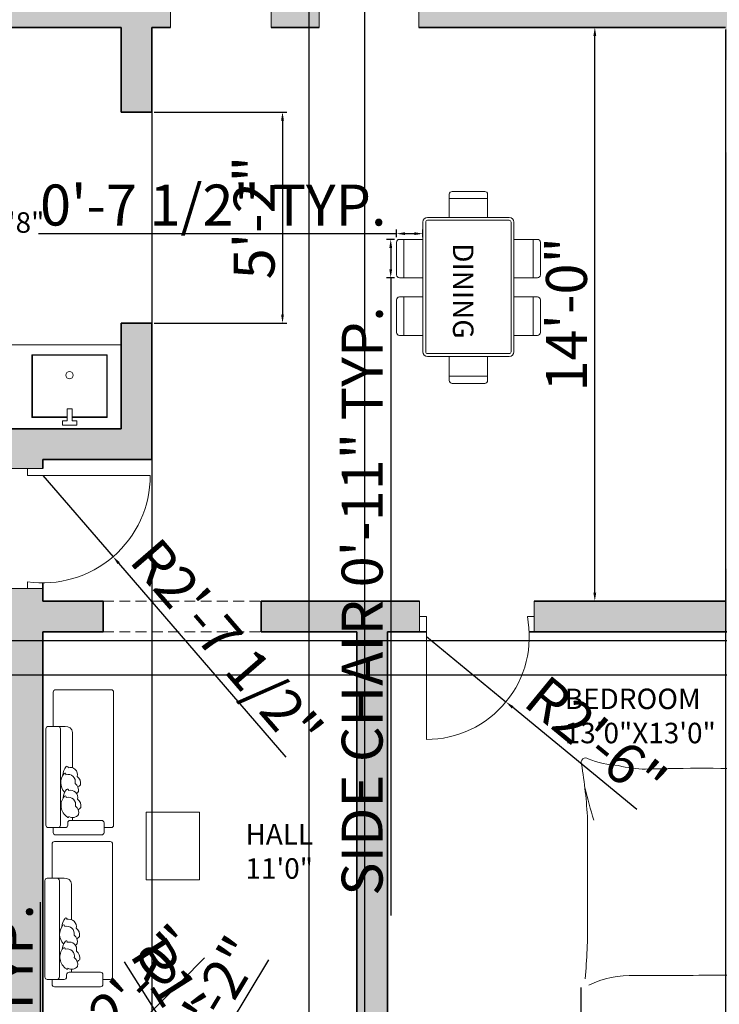
# Model space of a CAD drawing. Units: inches. Extents: x 995 to 1625, y 1005 to 1825.
# Tile 3 of 5: x 1174 to 1379, y 1232 to 1521. Entities that reach past the tile are written whole.
import ezdxf

# ---------------------------------------------------------------- set-up
doc = ezdxf.new("R2010")
doc.units = ezdxf.units.IN
doc.linetypes.add('HIDDEN2', pattern=[4.7625, 3.175, -1.5875])
for name, color, linetype, lineweight in [('A-ANNO-DIMS', 2, 'Continuous', 18), ('A-AREA-IDEN', 7, 'Continuous', 18), ('A-DOOR', 4, 'Continuous', 18), ('A-FLOR-CASE', 8, 'Continuous', 18), ('A-FLOR-FIXT', 9, 'Continuous', 18), ('A-FLOR-OVHD', 253, 'HIDDEN2', 18), ('A-FURN', 8, 'Continuous', 13), ('A-WALL', 7, 'Continuous', 35)]:
    doc.layers.add(name, color=color, linetype=linetype, lineweight=lineweight)
doc.layers.add('A-WALL-PATT', color=251, linetype='Continuous', lineweight=13, true_color=0x636466)
doc.styles.get("Standard").update_dxf_attribs({"font": 'arial.ttf'})
doc.dimstyles.new('ISO-25', dxfattribs={"dimtxt": 12, "dimasz": 2.5, "dimexe": 1.25, "dimexo": 0.625, "dimtad": 1, "dimdec": 0, "dimlunit": 3, "dimtxsty": 'Standard', "dimcen": 2.5, "dimadec": 0, "dimazin": 0, "dimtfac": 1, "dimtdec": 0, "dimtmove": 0, "dimatfit": 3, "dimfxl": 1, "dimarcsym": 0})

# ---------------------------------------------------------------- blocks, each defined once
blk = doc.blocks.new('BED-DOUBLE')
for p, q in [((13.64, 59.31), (35.36, 59.31)), ((15.43, 52.35), (14.57, 58.46)), ((14.57, 58.46), (18.38, 57.77)), ((18.38, 57.77), (20.29, 58.11)), ((20.29, 58.11), (24.62, 57.42)), ((24.45, 58.63), (23.23, 57.94)), ((27.57, 58.11), (24.45, 58.63)), ((31.38, 58.81), (27.57, 58.11)), ((31.35, 58.8), (31.75, 53.67)), ((33.52, 59.31), (33.52, 2.02)), ((35.36, 59.31), (35.36, 2.02)), ((16.62, 55.83), (15.82, 50.99)), ((24.62, 57.42), (27.91, 56.21)), ((15.82, 50.99), (15.43, 52.35)), ((31.73, 53.54), (31.38, 48.96)), ((31.75, 53.67), (31.73, 53.54)), ((15.82, 50.99), (15.3, 42.59)), ((31.38, 48.96), (30.17, 42.37)), ((-59.65, 45.42), (-59.65, 15.91)), ((30.86, 45.67), (31.73, 43.24)), ((15.3, 42.59), (15.97, 40.24)), ((31.73, 43.24), (32.59, 39.77)), ((15.97, 40.24), (15.49, 34.09)), ((15.86, 34.58), (17.17, 38.35)), ((32.59, 39.39), (32.42, 34.06)), ((32.59, 39.77), (32.59, 39.39)), ((15.86, 31.63), (15.86, 34.58)), ((33.11, 32.33), (26.7, 31.63)), ((32.42, 34.06), (33.11, 32.33)), ((18.31, 29.75), (15.1, 29.55)), ((15.1, 29.55), (15.29, 26.61)), ((19.07, 31.63), (15.86, 31.63)), ((20.52, 30.58), (18.31, 29.75)), ((21.33, 30.94), (19.07, 31.63)), ((22.07, 30.68), (20.52, 30.58)), ((22.89, 30.94), (21.33, 30.94)), ((25.92, 30.23), (22.07, 30.68)), ((26.7, 31.63), (22.89, 30.94)), ((32.37, 29.94), (25.92, 30.23)), ((31.78, 28.16), (32.37, 29.94)), ((14.51, 27.2), (6.73, 22.18)), ((15.29, 26.61), (16.83, 22.93)), ((32.29, 22.85), (31.78, 28.16)), ((11, 14.75), (14.51, 24.75)), ((16.62, 24.44), (15.82, 19.6)), ((6.73, 22.18), (1.35, 20.13)), ((31.66, 18.96), (32.31, 22.47)), ((32.31, 22.47), (32.29, 22.85)), ((1.35, 20.13), (-1.06, 19.76)), ((-1.06, 19.76), (-0.32, 16.79)), ((15.82, 19.6), (15.3, 11.2)), ((31.68, 13.23), (30.05, 19.72)), ((30.95, 16.48), (31.66, 18.96)), ((-0.32, 16.79), (0.79, 14.38)), ((8.59, 8.07), (11, 14.75)), ((0.79, 14.38), (1.35, 10.29)), ((32.31, 8.67), (31.68, 13.23)), ((1.35, 10.29), (1.72, 5.65)), ((15.3, 11.2), (15.97, 8.85)), ((15.97, 8.85), (15.49, 2.7)), ((32.29, 3.4), (32.41, 9.88)), ((32.41, 9.88), (32.31, 8.67)), ((5.99, 4.54), (8.59, 8.07)), ((25.46, 4.36), (28.67, 5.78)), ((1.72, 5.65), (1.35, 1.94)), ((2.09, 0.1), (5.99, 4.54)), ((15.49, 2.7), (19.25, 3.63)), ((19.25, 3.63), (21.17, 3.4)), ((21.17, 3.4), (25.46, 4.36)), ((25.36, 3.14), (24.1, 3.76)), ((28.44, 3.85), (25.36, 3.14)), ((32.29, 3.4), (28.44, 3.85)), ((0, 0), (2.09, 0.1, 4.64)), ((1.35, 1.94), (2.09, 0.1)), ((35.36, 2.02), (3.45, 2.02))]:
    blk.add_line(p, q)
for centre, radius, start, end in [((-60.22, 62.17), 1.31, 56.1736, 203.4781), ((-205.42, 37.79), 145.97, 2.9958, 9.4091), ((-48.9, 89.44), 28.25, 247.9751, 266.652), ((-41.99, 95.72), 35.53, 256.0648, 268.9113), ((-152.05, 42.19), 154.68, 351.7845, 6.9006), ((11.26, -38.62), 99.87, 88.7218, 95.604), ((-182.9, 37.87), 197.77, 356.0865, 6.7821), ((-25.32, -517.76), 578.22, 88.22771, 91.71854), ((-2.02, 264.05), 203.94, 268.4762, 271.0082), ((63.78, 84.12), 127.63, 193.3832, 197.7053), ((-1.14, 19.55), 0.221, 70.2464, 181.1377), ((33.58, 26.13), 35.55, 190.6617, 199.8806), ((-219.13, 14.14), 159.5, 354.4998, 0.6351), ((-6.68, 11.03), 7.46, 348.6608, 23.7384), ((43.33, 1.94), 43.38, 169.8763, 182.5657), ((-8.18, -155.03), 155.25, 86.9791, 93.8365), ((-46.97, -27.83), 27.65, 87.4714, 116.4681), ((-45.95, 5468.82), 5469.02, 270.00217, 270.28689)]:
    blk.add_arc(centre, radius, start, end)
blk = doc.blocks.new('DINING-CHAIR-SIDE')
for p, q in [((0, 0), (6.88, 0)), ((5.62, -11.24), (5.62, 0)), ((7.73, -0.84), (7.73, -10.4)), ((6.88, -11.24), (0, -11.24))]:
    blk.add_line(p, q)
for centre, start, end in [((6.88, -0.84), 0, 90), ((6.88, -10.4), 270, 0)]:
    blk.add_arc(centre, 0.843, start, end)
blk = doc.blocks.new('*D13')
at = {"layer": 'A-ANNO-DIMS', "color": 0, "lineweight": -2, "transparency": 16777216}
for p, q in [((1180.25, 1185.43), (1180.25, 1262.32)), ((1183.23, 1185.43), (1179, 1185.43)), ((1180.25, 1178.93), (1180.25, 1182.93)), ((1183.23, 1176.43), (1179, 1176.43))]:
    blk.add_line(p, q, dxfattribs=at)
at = {"layer": 'A-ANNO-DIMS', "color": 0, "transparency": 16777216}
for points in [[(1179.84, 1182.93), (1180.67, 1182.93), (1180.25, 1185.43)], [(1179.84, 1178.93), (1180.67, 1178.93), (1180.25, 1176.43)]]:
    blk.add_solid(points, dxfattribs=at)
at = {"layer": 'Defpoints', "color": 0, "transparency": 16777216}
for p in [(1180.25, 1185.43), (1183.85, 1185.43), (1183.85, 1176.43)]:
    blk.add_point(p, dxfattribs=at)
at = {"layer": 'A-ANNO-DIMS', "color": 0, "transparency": 16777216, "insert": (1173.5, 1225.13), "char_height": 12, "attachment_point": 5, "rotation": 90}
blk.add_mtext('0\'-9" TYP.', dxfattribs=at)
blk = doc.blocks.new('*D18')
at = {"layer": 'A-ANNO-DIMS', "color": 0, "lineweight": -2, "transparency": 16777216}
for p, q in [((1338.5, 1237.34), (1338.5, 1222.16)), ((1435.5, 1237.34), (1435.5, 1222.16)), ((1341, 1223.41), (1433, 1223.41)), ((1435.5, 1223.41), (1624.52, 1223.41))]:
    blk.add_line(p, q, dxfattribs=at)
at = {"layer": 'A-ANNO-DIMS', "color": 0, "transparency": 16777216}
for points in [[(1341, 1223.83), (1341, 1223), (1338.5, 1223.41)], [(1433, 1223.83), (1433, 1223), (1435.5, 1223.41)]]:
    blk.add_solid(points, dxfattribs=at)
at = {"layer": 'Defpoints', "color": 0, "transparency": 16777216}
for p in [(1338.5, 1237.96), (1435.5, 1237.96), (1435.5, 1223.41)]:
    blk.add_point(p, dxfattribs=at)
at = {"layer": 'A-ANNO-DIMS', "color": 0, "transparency": 16777216, "insert": (1531.26, 1230.25), "char_height": 12, "attachment_point": 5}
blk.add_mtext('DOUBLE BED 8\'-1" TYP.', dxfattribs=at)
blk = doc.blocks.new('*D20')
at = {"layer": 'A-ANNO-DIMS', "color": 0, "lineweight": -2, "transparency": 16777216}
for p, q in [((1283.89, 1456.35), (1281.57, 1456.35)), ((1282.82, 1453.85), (1282.82, 1447.61)), ((1283.89, 1445.11), (1281.57, 1445.11)), ((1282.82, 1445.11), (1282.82, 1258.35))]:
    blk.add_line(p, q, dxfattribs=at)
at = {"layer": 'A-ANNO-DIMS', "color": 0, "transparency": 16777216}
for points in [[(1282.41, 1453.85), (1283.24, 1453.85), (1282.82, 1456.35)], [(1282.41, 1447.61), (1283.24, 1447.61), (1282.82, 1445.11)]]:
    blk.add_solid(points, dxfattribs=at)
at = {"layer": 'Defpoints', "color": 0, "transparency": 16777216}
for p in [(1284.51, 1456.35), (1282.82, 1445.11), (1284.51, 1445.11)]:
    blk.add_point(p, dxfattribs=at)
at = {"layer": 'A-ANNO-DIMS', "color": 0, "transparency": 16777216, "insert": (1276, 1350.48), "char_height": 12, "attachment_point": 5, "rotation": 90}
blk.add_mtext('SIDE CHAIR 0\'-11" TYP.', dxfattribs=at)
blk = doc.blocks.new('*D21')
at = {"layer": 'A-ANNO-DIMS', "color": 0, "lineweight": -2, "transparency": 16777216}
for p, q in [((1284.51, 1456.97), (1284.51, 1459.28)), ((1292.24, 1456.97), (1292.24, 1459.28)), ((1284.51, 1458.03), (1179.65, 1458.03)), ((1289.74, 1458.03), (1287.01, 1458.03))]:
    blk.add_line(p, q, dxfattribs=at)
at = {"layer": 'A-ANNO-DIMS', "color": 0, "transparency": 16777216}
for points in [[(1287.01, 1458.45), (1287.01, 1457.62), (1284.51, 1458.03)], [(1289.74, 1458.45), (1289.74, 1457.62), (1292.24, 1458.03)]]:
    blk.add_solid(points, dxfattribs=at)
at = {"layer": 'Defpoints', "color": 0, "transparency": 16777216}
for p in [(1284.51, 1458.03), (1284.51, 1456.35), (1292.24, 1456.35)]:
    blk.add_point(p, dxfattribs=at)
at = {"layer": 'A-ANNO-DIMS', "color": 0, "transparency": 16777216, "insert": (1230.83, 1464.86), "char_height": 12, "attachment_point": 5}
blk.add_mtext('0\'-7 1/2" TYP.', dxfattribs=at)
blk = doc.blocks.new('*D26')
at = {"layer": 'A-ANNO-DIMS', "color": 0, "lineweight": -2, "transparency": 16777216}
for p, q in [((1076.49, 1338.88), (1486.37, 1338.88)), ((1485.12, 1336.38), (1485.12, 1331.38)), ((1076.49, 1328.88), (1486.37, 1328.88)), ((1485.12, 1328.88), (1485.12, 1283.91))]:
    blk.add_line(p, q, dxfattribs=at)
at = {"layer": 'A-ANNO-DIMS', "color": 0, "transparency": 16777216}
for points in [[(1484.7, 1336.38), (1485.53, 1336.38), (1485.12, 1338.88)], [(1484.7, 1331.38), (1485.53, 1331.38), (1485.12, 1328.88)]]:
    blk.add_solid(points, dxfattribs=at)
at = {"layer": 'Defpoints', "color": 0, "transparency": 16777216}
for p in [(1075.87, 1338.88), (1075.87, 1328.88), (1485.12, 1328.88)]:
    blk.add_point(p, dxfattribs=at)
at = {"layer": 'A-ANNO-DIMS', "color": 0, "transparency": 16777216, "insert": (1478.36, 1305.15), "char_height": 12, "attachment_point": 5, "rotation": 90}
blk.add_mtext('0\'-10"', dxfattribs=at)
blk = doc.blocks.new('*D29')
at = {"layer": 'A-ANNO-DIMS', "color": 0, "lineweight": -2, "transparency": 16777216}
for p, q in [((1380.24, 1518.43), (1341.37, 1518.43)), ((1342.62, 1352.93), (1342.62, 1515.93)), ((1380.24, 1350.43), (1341.37, 1350.43))]:
    blk.add_line(p, q, dxfattribs=at)
at = {"layer": 'A-ANNO-DIMS', "color": 0, "transparency": 16777216}
for points in [[(1342.2, 1515.93), (1343.03, 1515.93), (1342.62, 1518.43)], [(1342.2, 1352.93), (1343.03, 1352.93), (1342.62, 1350.43)]]:
    blk.add_solid(points, dxfattribs=at)
at = {"layer": 'Defpoints', "color": 0, "transparency": 16777216}
for p in [(1342.62, 1518.43), (1380.87, 1518.43), (1380.87, 1350.43)]:
    blk.add_point(p, dxfattribs=at)
at = {"layer": 'A-ANNO-DIMS', "color": 0, "transparency": 16777216, "insert": (1335.86, 1434.43), "char_height": 12, "attachment_point": 5, "rotation": 90}
blk.add_mtext('14\'-0"', dxfattribs=at)
blk = doc.blocks.new('*D30')
at = {"layer": 'A-ANNO-DIMS', "color": 0, "lineweight": -2, "transparency": 16777216}
for p, q in [((1212.87, 1517.8), (1212.87, 1015.27)), ((1380.87, 1517.8), (1380.87, 1015.27)), ((1215.37, 1016.52), (1378.37, 1016.52))]:
    blk.add_line(p, q, dxfattribs=at)
at = {"layer": 'A-ANNO-DIMS', "color": 0, "transparency": 16777216}
for points in [[(1215.37, 1016.93), (1215.37, 1016.1), (1212.87, 1016.52)], [(1378.37, 1016.93), (1378.37, 1016.1), (1380.87, 1016.52)]]:
    blk.add_solid(points, dxfattribs=at)
at = {"layer": 'Defpoints', "color": 0, "transparency": 16777216}
for p in [(1212.87, 1518.43), (1380.87, 1518.43), (1380.87, 1016.52)]:
    blk.add_point(p, dxfattribs=at)
at = {"layer": 'A-ANNO-DIMS', "color": 0, "transparency": 16777216, "insert": (1296.87, 1023.27), "char_height": 12, "attachment_point": 5}
blk.add_mtext('14\'-0"', dxfattribs=at)
blk = doc.blocks.new('*D31')
at = {"layer": 'A-ANNO-DIMS', "color": 0, "lineweight": -2, "transparency": 16777216}
for p, q in [((1213.49, 1493.65), (1252.37, 1493.65)), ((1251.12, 1491.15), (1251.12, 1434.33)), ((1213.49, 1431.83), (1252.37, 1431.83))]:
    blk.add_line(p, q, dxfattribs=at)
at = {"layer": 'A-ANNO-DIMS', "color": 0, "transparency": 16777216}
for points in [[(1250.7, 1491.15), (1251.53, 1491.15), (1251.12, 1493.65)], [(1250.7, 1434.33), (1251.53, 1434.33), (1251.12, 1431.83)]]:
    blk.add_solid(points, dxfattribs=at)
at = {"layer": 'Defpoints', "color": 0, "transparency": 16777216}
for p in [(1212.87, 1493.65), (1212.87, 1431.83), (1251.12, 1431.83)]:
    blk.add_point(p, dxfattribs=at)
at = {"layer": 'A-ANNO-DIMS', "color": 0, "transparency": 16777216, "insert": (1244.36, 1462.74), "char_height": 12, "attachment_point": 5, "rotation": 90}
blk.add_mtext('5\'-2"', dxfattribs=at)
blk = doc.blocks.new('*D32')
at = {"layer": 'A-ANNO-DIMS', "color": 0, "lineweight": -2, "transparency": 16777216}
for p, q in [((1180.87, 1340.8), (1180.87, 1015.27)), ((1272.87, 1340.8), (1272.87, 1015.27)), ((1183.37, 1016.52), (1270.37, 1016.52))]:
    blk.add_line(p, q, dxfattribs=at)
at = {"layer": 'A-ANNO-DIMS', "color": 0, "transparency": 16777216}
for points in [[(1183.37, 1016.93), (1183.37, 1016.1), (1180.87, 1016.52)], [(1270.37, 1016.93), (1270.37, 1016.1), (1272.87, 1016.52)]]:
    blk.add_solid(points, dxfattribs=at)
at = {"layer": 'Defpoints', "color": 0, "transparency": 16777216}
for p in [(1180.87, 1341.43), (1272.87, 1341.43), (1272.87, 1016.52)]:
    blk.add_point(p, dxfattribs=at)
at = {"layer": 'A-ANNO-DIMS', "color": 0, "transparency": 16777216, "insert": (1226.87, 1023.27), "char_height": 12, "attachment_point": 5}
blk.add_mtext('7\'-8"', dxfattribs=at)
blk = doc.blocks.new('*D37')
at = {"layer": 'A-ANNO-DIMS', "color": 0, "lineweight": -2, "transparency": 16777216}
for p, q in [((1258.87, 1658.8), (1258.87, 1015.27)), ((1275.16, 1658.8), (1275.16, 1015.27)), ((1261.37, 1016.52), (1272.66, 1016.52)), ((1275.16, 1016.52), (1337.64, 1016.52))]:
    blk.add_line(p, q, dxfattribs=at)
at = {"layer": 'A-ANNO-DIMS', "color": 0, "transparency": 16777216}
for points in [[(1261.37, 1016.93), (1261.37, 1016.1), (1258.87, 1016.52)], [(1272.66, 1016.93), (1272.66, 1016.1), (1275.16, 1016.52)]]:
    blk.add_solid(points, dxfattribs=at)
at = {"layer": 'Defpoints', "color": 0, "transparency": 16777216}
for p in [(1258.87, 1659.43), (1275.16, 1659.43), (1275.16, 1016.52)]:
    blk.add_point(p, dxfattribs=at)
at = {"layer": 'A-ANNO-DIMS', "color": 0, "transparency": 16777216, "insert": (1307.65, 1023.35), "char_height": 12, "attachment_point": 5}
blk.add_mtext('1\'-4 1/2"', dxfattribs=at)
blk = doc.blocks.new('*D44')
at = {"layer": 'A-ANNO-DIMS', "color": 0, "lineweight": -2, "transparency": 16777216}
for p, q in [((1180.93, 1387.24), (1201.48, 1363.45)), ((1252.21, 1304.73), (1203.12, 1361.56))]:
    blk.add_line(p, q, dxfattribs=at)
at = {"layer": 'A-ANNO-DIMS', "color": 0, "transparency": 16777216}
blk.add_solid([(1203.43, 1361.83), (1202.8, 1361.28), (1201.48, 1363.45)], dxfattribs=at)
at = {"layer": 'Defpoints', "color": 0, "transparency": 16777216}
for p in [(1180.93, 1387.24), (1201.48, 1363.45)]:
    blk.add_point(p, dxfattribs=at)
at = {"layer": 'A-ANNO-DIMS', "color": 0, "transparency": 16777216, "insert": (1233.65, 1336.66), "char_height": 12, "attachment_point": 5, "rotation": 310.8272}
blk.add_mtext('R2\'-7 1/2"', dxfattribs=at)
blk = doc.blocks.new('*D45')
at = {"layer": 'A-ANNO-DIMS', "color": 0, "lineweight": -2, "transparency": 16777216}
for p, q in [((1293.29, 1340.07), (1316.58, 1320.94)), ((1354.94, 1289.44), (1318.51, 1319.35))]:
    blk.add_line(p, q, dxfattribs=at)
at = {"layer": 'A-ANNO-DIMS', "color": 0, "transparency": 16777216}
blk.add_solid([(1318.78, 1319.67), (1318.25, 1319.03), (1316.58, 1320.94)], dxfattribs=at)
at = {"layer": 'Defpoints', "color": 0, "transparency": 16777216}
for p in [(1293.29, 1340.07), (1316.58, 1320.94)]:
    blk.add_point(p, dxfattribs=at)
at = {"layer": 'A-ANNO-DIMS', "color": 0, "transparency": 16777216, "insert": (1341.98, 1308.82), "char_height": 12, "attachment_point": 5, "rotation": 320.6072}
blk.add_mtext('R2\'-6"', dxfattribs=at)
blk = doc.blocks.new('*D50')
at = {"layer": 'A-ANNO-DIMS', "color": 0, "lineweight": -2, "transparency": 16777216}
for p, q in [((1228.3, 1245.97), (1195.09, 1212.53)), ((1176.53, 1193.84), (1193.33, 1210.75))]:
    blk.add_line(p, q, dxfattribs=at)
at = {"layer": 'A-ANNO-DIMS', "color": 0, "transparency": 16777216}
blk.add_solid([(1194.79, 1212.82), (1195.38, 1212.23), (1193.33, 1210.75)], dxfattribs=at)
at = {"layer": 'Defpoints', "color": 0, "transparency": 16777216}
for p in [(1193.33, 1210.75), (1176.53, 1193.84)]:
    blk.add_point(p, dxfattribs=at)
at = {"layer": 'A-ANNO-DIMS', "color": 0, "transparency": 16777216, "insert": (1207.79, 1234.89), "char_height": 12, "attachment_point": 5, "rotation": 45.1957}
blk.add_mtext('R2\'-0"', dxfattribs=at)
blk = doc.blocks.new('*D54')
at = {"layer": 'A-ANNO-DIMS', "color": 0, "lineweight": -2, "transparency": 16777216}
for p, q in [((1246.99, 1245.39), (1222.61, 1205.06)), ((1214.11, 1191), (1221.31, 1202.92))]:
    blk.add_line(p, q, dxfattribs=at)
at = {"layer": 'A-ANNO-DIMS', "color": 0, "transparency": 16777216}
blk.add_solid([(1222.25, 1205.27), (1222.96, 1204.84), (1221.31, 1202.92)], dxfattribs=at)
at = {"layer": 'Defpoints', "color": 0, "transparency": 16777216}
for p in [(1221.31, 1202.92), (1214.11, 1191)]:
    blk.add_point(p, dxfattribs=at)
at = {"layer": 'A-ANNO-DIMS', "color": 0, "transparency": 16777216, "insert": (1229.75, 1229.74), "char_height": 12, "attachment_point": 5, "rotation": 58.8445}
blk.add_mtext('R1\'-2"', dxfattribs=at)
blk = doc.blocks.new('*D55')
at = {"layer": 'A-ANNO-DIMS', "color": 0, "lineweight": -2, "transparency": 16777216}
for p, q in [((1204.75, 1244.87), (1229.92, 1205.02)), ((1238.24, 1191.86), (1231.26, 1202.91))]:
    blk.add_line(p, q, dxfattribs=at)
at = {"layer": 'A-ANNO-DIMS', "color": 0, "transparency": 16777216}
blk.add_solid([(1230.28, 1205.24), (1229.57, 1204.8), (1231.26, 1202.91)], dxfattribs=at)
at = {"layer": 'Defpoints', "color": 0, "transparency": 16777216}
for p in [(1231.26, 1202.91), (1238.24, 1191.86)]:
    blk.add_point(p, dxfattribs=at)
at = {"layer": 'A-ANNO-DIMS', "color": 0, "transparency": 16777216, "insert": (1222.29, 1229.55), "char_height": 12, "attachment_point": 5, "rotation": 302.2824}
blk.add_mtext('R1\'-1"', dxfattribs=at)

msp = doc.modelspace()

# ---------------------------------------------------------------- hatches: boundary and pattern name
at = {"layer": 'A-WALL-PATT'}
h = msp.add_hatch(color=256, dxfattribs=at)
h.dxf.hatch_style = 1
h.paths.add_polyline_path([(1446.87, 1737.43), (1066.87, 1737.43), (1066.87, 1718.28), (1075.87, 1718.28), (1075.87, 1728.43), (1171.87, 1728.43), (1171.87, 1668.43), (1165.05, 1668.43), (1165.05, 1659.43), (1219.13, 1659.43), (1219.13, 1663.93), (1219.13, 1668.43), (1180.87, 1668.43), (1180.87, 1691.88), (1180.87, 1728.43), (1249.87, 1728.43), (1258.87, 1728.43), (1332.87, 1728.43), (1332.87, 1668.43), (1311.16, 1668.43), (1311.16, 1659.43), (1346.35, 1659.43), (1346.35, 1663.93), (1346.35, 1668.43), (1341.87, 1668.43), (1341.87, 1728.43), (1437.87, 1728.43), (1437.87, 1715.56), (1446.87, 1715.56)])
h.paths.add_polyline_path([(1135.58, 1663.93), (1135.58, 1668.43), (1075.87, 1668.43), (1075.87, 1694.28), (1066.87, 1694.28), (1066.87, 1619.54), (1075.87, 1619.54), (1075.87, 1659.43), (1135.58, 1659.43)])
h.paths.add_polyline_path([(1258.87, 1659.43), (1275.16, 1659.43), (1275.16, 1663.93), (1275.16, 1668.43), (1258.87, 1668.43), (1249.87, 1668.43), (1243.74, 1668.43), (1243.74, 1659.43), (1249.87, 1659.43), (1249.87, 1527.43), (1247.75, 1527.43), (1247.75, 1518.43), (1261.81, 1518.43), (1261.81, 1527.43), (1258.87, 1527.43)])
h.paths.add_polyline_path([(1446.87, 1691.56), (1437.87, 1691.56), (1437.87, 1668.43), (1372.6, 1668.43), (1372.6, 1659.43), (1437.87, 1659.43), (1437.87, 1627.58), (1446.87, 1627.58)])
h.paths.add_polyline_path([(1446.87, 1567.58), (1437.87, 1567.58), (1437.87, 1527.43), (1291.03, 1527.43), (1291.03, 1518.43), (1380.87, 1518.43), (1380.87, 1508.92), (1389.87, 1508.92), (1389.87, 1518.43), (1437.87, 1518.43), (1437.87, 1501.62), (1446.87, 1501.62)])
h.paths.add_polyline_path([(1446.87, 1477.62), (1437.87, 1477.62), (1437.87, 1429.75), (1446.87, 1429.75)])
h.paths.add_polyline_path([(1389.87, 1441.43), (1437.87, 1441.43), (1437.87, 1450.43), (1389.87, 1450.43), (1389.87, 1481.88), (1385.37, 1481.88), (1380.87, 1481.88), (1380.87, 1385.88), (1389.87, 1385.88)])
h.paths.add_polyline_path([(1446.87, 1405.75), (1437.87, 1405.75), (1437.87, 1350.43), (1427.33, 1350.43), (1389.87, 1350.43), (1389.87, 1359.9), (1380.87, 1359.9), (1380.87, 1350.43), (1324.85, 1350.43), (1324.85, 1341.43), (1437.87, 1341.43), (1437.87, 1303.84), (1446.87, 1303.84)])
h.paths.add_polyline_path([(1311.82, 1209.43), (1281.87, 1209.43), (1281.87, 1341.43), (1291.29, 1341.43), (1291.29, 1345.93), (1291.29, 1350.43), (1244.83, 1350.43), (1244.83, 1341.43), (1272.87, 1341.43), (1272.87, 1185.43), (1268.73, 1185.43), (1268.73, 1176.43), (1272.87, 1176.43), (1281.87, 1176.43), (1281.87, 1200.43), (1311.82, 1200.43), (1311.82, 1204.93)])
h.paths.add_polyline_path([(1446.87, 1243.84), (1437.87, 1243.84), (1437.87, 1209.43), (1371.82, 1209.43), (1371.82, 1200.43), (1437.87, 1200.43), (1437.87, 1107.43), (1446.87, 1107.43)])
h.paths.add_polyline_path([(1212.11, 1185.43), (1207.85, 1185.43), (1207.85, 1176.43), (1212.11, 1176.43)], flags=17)
h.paths.add_polyline_path([(1244.73, 1185.43), (1240.24, 1185.43), (1240.24, 1176.43), (1244.73, 1176.43), (1244.73, 1180.93)])
h.paths.add_polyline_path([(1183.85, 1180.93), (1183.85, 1185.43), (1180.87, 1185.43), (1180.87, 1191.84), (1171.87, 1191.84), (1171.87, 1176.43), (1180.87, 1176.43), (1183.85, 1176.43)], flags=17)
h.paths.add_polyline_path([(1180.87, 1341.43), (1198.57, 1341.43), (1198.57, 1350.43), (1180.87, 1350.43), (1180.87, 1354.13), (1176.37, 1354.13), (1171.87, 1354.13), (1171.87, 1341.43), (1171.87, 1219.68), (1180.87, 1219.68)], flags=17)
h.paths.add_polyline_path([(1075.87, 1391.93), (1171.87, 1391.93), (1171.87, 1389.24), (1180.87, 1389.24), (1180.87, 1391.93), (1212.87, 1391.93), (1212.87, 1431.83), (1203.87, 1431.83), (1203.87, 1400.93), (1075.87, 1400.93), (1075.87, 1446.29), (1066.87, 1446.29), (1066.87, 1107.43), (1075.87, 1107.43)])
h.paths.add_polyline_path([(1218.33, 1527.43), (1075.87, 1527.43), (1075.87, 1559.54), (1066.87, 1559.54), (1066.87, 1482.29), (1075.87, 1482.29), (1075.87, 1518.43), (1203.87, 1518.43), (1203.87, 1493.65), (1212.87, 1493.65), (1212.87, 1518.43), (1218.33, 1518.43), (1218.33, 1522.93)])
h.paths.add_polyline_path([(1297.68, 1457.37), (1297.68, 1425.03), (1310.04, 1425.03), (1310.04, 1457.37)], flags=9)
h.paths.add_polyline_path([(1154.86, 1054.62), (1346.22, 1054.62), (1346.22, 1079.35), (1154.86, 1079.35)], flags=9)
h.paths.add_polyline_path([(1237.85, 1265.85), (1262.06, 1265.85), (1262.06, 1288.24), (1237.85, 1288.24)], flags=9)
h.paths.add_polyline_path([(1331.39, 1305.41), (1378, 1305.41), (1378, 1327.8), (1331.39, 1327.8)], flags=25)
h.paths.add_polyline_path([(1395.38, 1378.18), (1431.86, 1378.18), (1431.86, 1400.57), (1395.38, 1400.57)], flags=25)
h.paths.add_polyline_path([(1406.34, 1460.18), (1434.48, 1460.18), (1434.48, 1472.55), (1406.34, 1472.55)], flags=25)
h.paths.add_polyline_path([(1134.66, 1454.9), (1180.38, 1454.9), (1180.38, 1477.29), (1134.66, 1477.29)], flags=9)
h.paths.add_polyline_path([(1109.63, 1626.32), (1156.23, 1626.32), (1156.23, 1648.71), (1109.63, 1648.71)], flags=9)
h.paths.add_polyline_path([(1275.64, 1623.22), (1322.25, 1623.22), (1322.25, 1645.61), (1275.64, 1645.61)], flags=9)
h.paths.add_polyline_path([(1347.7, 1693.6), (1384.09, 1693.6), (1384.09, 1715.99), (1347.7, 1715.99)], flags=25)
h.paths.add_polyline_path([(1254.21, 1701.46), (1308.94, 1701.46), (1308.94, 1723.85), (1254.21, 1723.85)], flags=25)
h.paths.add_polyline_path([(1107.35, 1692.25), (1143.74, 1692.25), (1143.74, 1714.64), (1107.35, 1714.64)], flags=25)

# ---------------------------------------------------------------- linework, layer by layer
at = {"layer": 'A-DOOR'}
for p, q in [((1218.33, 1527.43), (1218.33, 1518.43)), ((1247.75, 1527.43), (1247.75, 1518.43)), ((1261.81, 1527.43), (1261.81, 1518.43)), ((1291.03, 1527.43), (1291.03, 1518.43)), ((1218.33, 1518.43), (1218.33, 1522.93)), ((1291.03, 1518.43), (1291.03, 1522.93)), ((1171.87, 1389.24), (1180.87, 1389.24)), ((1180.87, 1389.24), (1176.37, 1389.24)), ((1176.37, 1389.24), (1176.37, 1387.24)), ((1176.37, 1387.24), (1212.37, 1387.24)), ((1176.37, 1354.13), (1176.37, 1356.13)), ((1171.87, 1354.13), (1180.87, 1354.13)), ((1180.87, 1354.13), (1176.37, 1354.13)), ((1291.29, 1350.43), (1291.29, 1341.43)), ((1324.85, 1350.43), (1324.85, 1341.43)), ((1291.29, 1341.43), (1291.29, 1345.93)), ((1291.29, 1345.93), (1293.29, 1345.93)), ((1293.29, 1345.93), (1293.29, 1309.93)), ((1324.85, 1345.93), (1322.85, 1345.93)), ((1324.85, 1341.43), (1324.85, 1345.93))]:
    msp.add_line(p, q, dxfattribs=at)
for centre, radius, start, end in [((1180.93, 1387.24), 31.44, 261.654, 0), ((1293.29, 1340.07), 30.14, 270, 11.2144)]:
    msp.add_arc(centre, radius, start, end, dxfattribs=at)
at = {"layer": 'A-FLOR-CASE'}
msp.add_line((1109.19, 1425.49), (1203.87, 1425.49), dxfattribs=at)
at = {"layer": 'A-FLOR-FIXT'}
for p, q in [((1177.86, 1404.4), (1177.86, 1422.54)), ((1177.86, 1422.54), (1177.86, 1422.41)), ((1177.86, 1422.41), (1199.76, 1422.41)), ((1199.76, 1422.41), (1199.66, 1422.41)), ((1199.66, 1422.41), (1199.66, 1404.25)), ((1188.07, 1404.4), (1177.69, 1404.4)), ((1177.69, 1404.4), (1177.86, 1404.4)), ((1188.07, 1406.78), (1189.45, 1406.78)), ((1188.07, 1404.25), (1188.07, 1404.4)), ((1199.66, 1404.36), (1189.45, 1404.36)), ((1199.66, 1404.25), (1199.66, 1404.36))]:
    msp.add_line(p, q, dxfattribs=at)
for points in [[(1188.07, 1404.25), (1177.69, 1404.25), (1177.69, 1422.54), (1199.76, 1422.54), (1199.76, 1404.25), (1189.45, 1404.25)], [(1188.07, 1403.24), (1188.07, 1406.78)], [(1189.45, 1406.78), (1189.45, 1403.24)], [(1189.45, 1403.24), (1190.86, 1403.24), (1190.86, 1401.96), (1186.62, 1401.96), (1186.62, 1403.24), (1188.07, 1403.24)]]:
    msp.add_lwpolyline(points, dxfattribs=at)
msp.add_circle((1188.71, 1416.6), 1.04, dxfattribs=at)
at = {"layer": 'A-FLOR-OVHD'}
for p, q in [((1198.57, 1350.43), (1244.83, 1350.43)), ((1198.57, 1341.43), (1244.83, 1341.43))]:
    msp.add_line(p, q, dxfattribs=at)
at = {"layer": 'A-FURN'}
for p, q in [((1310.36, 1470.39), (1300.81, 1470.39)), ((1299.96, 1469.55), (1299.96, 1462.81)), ((1299.96, 1468.29), (1311.2, 1468.29)), ((1311.2, 1462.81), (1311.2, 1469.55)), ((1293.64, 1462.81), (1317.52, 1462.81)), ((1293.64, 1461.97), (1317.52, 1461.97)), ((1292.24, 1423.47), (1292.24, 1461.4)), ((1293.08, 1423.47), (1293.08, 1461.4)), ((1318.09, 1461.4), (1318.09, 1423.47)), ((1318.93, 1461.4), (1318.93, 1423.47)), ((1317.52, 1422.91), (1293.64, 1422.91)), ((1317.52, 1422.07), (1293.64, 1422.07)), ((1299.96, 1415.05), (1299.96, 1422.07)), ((1311.2, 1422.07), (1311.2, 1415.05)), ((1299.96, 1416.31), (1311.2, 1416.31)), ((1310.36, 1414.2), (1300.81, 1414.2))]:
    msp.add_line(p, q, dxfattribs=at)
at = {"layer": 'A-FURN', "ltscale": 0.03}
for points in [[(1200.94, 1324.49), (1184.65, 1324.49, 0.414214), (1183.94, 1323.78), (1183.94, 1313.76), (1182.52, 1313.76, 0.414214), (1181.81, 1313.05), (1181.81, 1284.81, 0.414214), (1182.52, 1284.11), (1183.94, 1284.11), (1183.94, 1282.69, 0.414214), (1184.65, 1281.98), (1198.11, 1281.98, 0.414214), (1198.82, 1282.69), (1198.82, 1284.11), (1200.94, 1284.11, 0.414214), (1201.65, 1284.81), (1201.65, 1323.78, 0.414214), (1200.94, 1324.49)], [(1200.62, 1280.05), (1184.33, 1280.05, 0.414214), (1183.62, 1279.34), (1183.62, 1269.32), (1182.2, 1269.32, 0.414214), (1181.49, 1268.61), (1181.49, 1240.37, 0.414214), (1182.2, 1239.67), (1183.62, 1239.67), (1183.62, 1238.25, 0.414214), (1184.33, 1237.54), (1197.79, 1237.54, 0.414214), (1198.5, 1238.25), (1198.5, 1239.67), (1200.62, 1239.67, 0.414214), (1201.33, 1240.37), (1201.33, 1279.34, 0.414214), (1200.62, 1280.05)]]:
    msp.add_lwpolyline(points, format="xyb", dxfattribs=at)
at = {"layer": 'A-FURN'}
for points in [[(1183.94, 1313.76), (1182.52, 1313.76, 0.414214), (1181.81, 1313.05), (1181.81, 1284.81, 0.414214), (1182.52, 1284.11), (1185.36, 1284.11, 0.414214), (1186.07, 1284.81), (1186.07, 1313.05, 0.414214), (1185.36, 1313.76), (1183.94, 1313.76)], [(1183.62, 1269.32), (1182.2, 1269.32, 0.414214), (1181.49, 1268.61), (1181.49, 1240.37, 0.414214), (1182.2, 1239.67), (1185.04, 1239.67, 0.414214), (1185.74, 1240.37), (1185.74, 1268.61, 0.414214), (1185.04, 1269.32), (1183.62, 1269.32)]]:
    msp.add_lwpolyline(points, format="xyb", close=True, dxfattribs=at)
for points in [[(1189.61, 1301.63), (1189.61, 1312.01, 0.413601), (1187.48, 1313.76), (1183.94, 1313.76)], [(1183.94, 1284.11), (1183.94, 1282.69, 0.414214), (1184.65, 1281.98), (1198.11, 1281.98, 0.414214), (1198.82, 1282.69), (1198.82, 1285.52, 0.414214), (1198.11, 1286.23), (1188.9, 1286.23, 0.414214), (1188.19, 1285.52), (1188.19, 1284.81, -0.414214), (1187.48, 1284.11), (1185.36, 1284.11)], [(1189.29, 1257.19), (1189.29, 1267.57, 0.413601), (1187.16, 1269.32), (1183.62, 1269.32)], [(1183.62, 1239.67), (1183.62, 1238.25, 0.414214), (1184.33, 1237.54), (1197.79, 1237.54, 0.414214), (1198.5, 1238.25), (1198.5, 1241.08, 0.414214), (1197.79, 1241.79), (1188.58, 1241.79, 0.414214), (1187.87, 1241.08), (1187.87, 1240.37, -0.414214), (1187.16, 1239.67), (1185.04, 1239.67)]]:
    msp.add_lwpolyline(points, format="xyb", dxfattribs=at)
for points in [[(1189.61, 1286.23), (1189.61, 1287.09)], [(1189.29, 1241.79), (1189.29, 1242.65)]]:
    msp.add_lwpolyline(points, dxfattribs=at)
msp.add_lwpolyline([(1211.17, 1288.63), (1226.83, 1288.63), (1226.83, 1268.83), (1211.17, 1268.83)], close=True, dxfattribs=at)
for centre, radius, start, end in [((1300.81, 1469.55), 0.843, 90, 180), ((1310.36, 1469.55), 0.843, 0, 90), ((1293.64, 1461.4), 1.4, 90, 180), ((1293.64, 1461.4), 0.562, 90, 180), ((1317.52, 1461.4), 1.4, 0, 90), ((1317.52, 1461.4), 0.562, 0, 90), ((1293.64, 1423.47), 1.4, 180, 270), ((1293.64, 1423.47), 0.562, 180, 270), ((1317.52, 1423.47), 1.4, 270, 0), ((1317.52, 1423.47), 0.562, 270, 0), ((1300.81, 1415.05), 0.843, 180, 270), ((1310.36, 1415.05), 0.843, 270, 0), ((1190.88, 1299.35), 4.11, 139.9254, 177.8787), ((1187.98, 1301.77), 0.337, 339.3279, 136.5017), ((1188.92, 1299.61), 2.13, 345.9033, 107.0512), ((1190.26, 1297.32), 4.11, 139.9254, 223.5565), ((1187.35, 1299.74), 0.337, 339.3279, 136.5017), ((1188.29, 1297.58), 2.13, 345.9033, 107.0512), ((1189.58, 1297.15), 2.4, 347.911, 54.2645), ((1190.97, 1292.68), 4.11, 139.9254, 177.8787), ((1188.07, 1295.09), 0.337, 339.3279, 136.5017), ((1189.01, 1292.94), 2.13, 345.9033, 107.0512), ((1188.96, 1295.12), 2.4, 347.911, 54.2645), ((1189.57, 1295.95), 2.18, 303.4416, 322.3806), ((1190.2, 1297.98), 2.18, 296.6318, 322.3806), ((1190.35, 1290.65), 4.11, 139.9254, 237.1968), ((1187.44, 1293.06), 0.337, 339.3279, 136.5017), ((1188.38, 1290.91), 2.13, 345.9033, 107.0512), ((1189.67, 1290.47), 2.4, 347.911, 54.2645), ((1189.05, 1288.44), 2.4, 347.911, 54.2645), ((1190.29, 1291.31), 2.18, 296.6318, 322.3806), ((1188.3, 1287.36), 0.254, 223.5349, 6.6534), ((1189.66, 1289.27), 2.18, 239.5514, 322.3806), ((1190.56, 1254.91), 4.11, 139.9254, 177.8787), ((1187.66, 1257.33), 0.337, 339.3279, 136.5017), ((1188.59, 1255.17), 2.13, 345.9033, 107.0512), ((1189.93, 1252.88), 4.11, 139.9254, 223.5565), ((1187.03, 1255.3), 0.337, 339.3279, 136.5017), ((1187.97, 1253.14), 2.13, 345.9033, 107.0512), ((1189.26, 1252.71), 2.4, 347.911, 54.2645), ((1188.64, 1250.68), 2.4, 347.911, 54.2645), ((1189.87, 1253.54), 2.18, 296.6318, 322.3806), ((1190.02, 1246.2), 4.11, 139.9254, 237.1968), ((1190.65, 1248.24), 4.11, 139.9254, 177.8787), ((1187.12, 1248.62), 0.337, 339.3279, 136.5017), ((1188.06, 1246.47), 2.13, 345.9033, 107.0512), ((1187.75, 1250.65), 0.337, 339.3279, 136.5017), ((1188.68, 1248.5), 2.13, 345.9033, 107.0512), ((1189.25, 1251.51), 2.18, 303.4416, 322.3806), ((1188.73, 1244), 2.4, 347.911, 54.2645), ((1189.35, 1246.03), 2.4, 347.911, 54.2645), ((1189.96, 1246.87), 2.18, 296.6318, 322.3806), ((1187.98, 1242.92), 0.254, 223.5349, 6.6534), ((1189.34, 1244.83), 2.18, 239.5514, 322.3806)]:
    msp.add_arc(centre, radius, start, end, dxfattribs=at)
at = {"layer": 'A-WALL'}
for p, q in [((1075.87, 1518.43), (1203.87, 1518.43)), ((1203.87, 1518.43), (1203.87, 1493.65)), ((1212.87, 1518.43), (1212.87, 1493.65)), ((1212.87, 1518.43), (1218.33, 1518.43)), ((1247.75, 1518.43), (1261.81, 1518.43)), ((1291.03, 1518.43), (1380.87, 1518.43)), ((1203.87, 1493.65), (1212.87, 1493.65)), ((1203.87, 1431.83), (1212.87, 1431.83)), ((1203.87, 1431.83), (1203.87, 1400.93)), ((1212.87, 1431.83), (1212.87, 1391.93)), ((1203.87, 1400.93), (1075.87, 1400.93)), ((1180.87, 1389.24), (1180.87, 1391.93)), ((1180.87, 1391.93), (1212.87, 1391.93)), ((1180.87, 1355.8), (1180.87, 1350.43)), ((1180.87, 1350.43), (1198.57, 1350.43)), ((1198.57, 1350.43), (1198.57, 1341.43)), ((1244.83, 1350.43), (1244.83, 1341.43)), ((1244.83, 1350.43), (1291.29, 1350.43)), ((1324.85, 1350.43), (1380.87, 1350.43)), ((1180.87, 1341.43), (1180.87, 1217.28)), ((1180.87, 1341.43), (1198.57, 1341.43)), ((1244.83, 1341.43), (1272.87, 1341.43)), ((1272.87, 1341.43), (1272.87, 1185.43)), ((1281.87, 1341.43), (1281.87, 1209.43)), ((1281.87, 1341.43), (1293.29, 1341.43)), ((1323.4, 1341.43), (1437.87, 1341.43))]:
    msp.add_line(p, q, dxfattribs=at)

# ---------------------------------------------------------------- block references
at = {"layer": 'A-FURN', "rotation": 180}
for p in [(1292.24, 1445.11), (1292.24, 1428.25)]:
    msp.add_blockref('DINING-CHAIR-SIDE', p, dxfattribs=at)
at = {"layer": 'A-FURN'}
for name, p in [('DINING-CHAIR-SIDE', (1318.93, 1456.35)), ('DINING-CHAIR-SIDE', (1318.93, 1439.49)), ('BED-DOUBLE', (1400.14, 1241.04))]:
    msp.add_blockref(name, p, dxfattribs=at)

# ---------------------------------------------------------------- texts
at = {"layer": 'A-AREA-IDEN', "char_height": 6, "attachment_point": 1}
for s, width, insert in [('KITCHEN\\P14\'0"X10\'8"', 168.4596, (1137.08, 1474.3)), ('BEDROOM\\P13\'0"X13\'0"', 197.611, (1333.8, 1324.82)), ('HALL\\P11\'0"', 79.6045, (1240.26, 1285.16))]:
    msp.add_mtext_dynamic_manual_height_columns(s, width=width, gutter_width=12.5, heights=[0], dxfattribs=dict(at, insert=insert))
at = {"layer": 'A-AREA-IDEN', "insert": (1307.06, 1455.22), "char_height": 6, "attachment_point": 1, "rotation": 270}
msp.add_mtext_dynamic_manual_height_columns('DINING', width=109.2996, gutter_width=12.5, heights=[0], dxfattribs=at)

# ---------------------------------------------------------------- dimensions: what is measured, and where the dimension line sits
at = {"layer": 'A-ANNO-DIMS'}
for base, p1, p2, picture, middle in [((1275.16, 1016.52), (1258.87, 1659.43), (1275.16, 1659.43), '*D37', (1307.65, 1023.35)), ((1380.87, 1016.52), (1212.87, 1518.43), (1380.87, 1518.43), '*D30', (1296.87, 1023.27)), ((1272.87, 1016.52), (1180.87, 1341.43), (1272.87, 1341.43), '*D32', (1226.87, 1023.27))]:
    dim = msp.add_linear_dim(base=base, p1=p1, p2=p2, dimstyle='ISO-25', override={"dimdec": 1, "dimlfac": 1, "dimrnd": 0, "dimzin": 1, "dimdsep": 46, "dimlunit": 4, "dimfrac": 2}, dxfattribs=at)
    dim.commit()
    dim.dimension.update_dxf_attribs({"geometry": picture, "text_midpoint": middle})
for base, p1, p2, angle, picture, middle in [((1342.62, 1518.43), (1380.87, 1350.43), (1380.87, 1518.43), 90, '*D29', (1335.86, 1434.43)), ((1251.12, 1431.83), (1212.87, 1493.65), (1212.87, 1431.83), 270, '*D31', (1244.36, 1462.74)), ((1485.12, 1328.88), (1075.87, 1338.88), (1075.87, 1328.88), 90, '*D26', (1478.36, 1305.15))]:
    dim = msp.add_linear_dim(base=base, p1=p1, p2=p2, angle=angle, dimstyle='ISO-25', override={"dimdec": 1, "dimlfac": 1, "dimrnd": 0, "dimzin": 1, "dimdsep": 46, "dimlunit": 4, "dimfrac": 2}, dxfattribs=at)
    dim.commit()
    dim.dimension.update_dxf_attribs({"geometry": picture, "text_midpoint": middle})
for base, p1, p2, angle, text, picture, middle in [((1284.51, 1458.03), (1292.24, 1456.35), (1284.51, 1456.35), 180, '<> TYP.', '*D21', (1230.83, 1464.86)), ((1282.82, 1445.11), (1284.51, 1456.35), (1284.51, 1445.11), 270, 'SIDE CHAIR <> TYP.', '*D20', (1276, 1350.48)), ((1180.25, 1185.43), (1183.85, 1176.43), (1183.85, 1185.43), 90, '<> TYP.', '*D13', (1173.5, 1225.13))]:
    dim = msp.add_linear_dim(base=base, p1=p1, p2=p2, angle=angle, text=text, dimstyle='ISO-25', override={"dimdec": 1, "dimlfac": 1, "dimrnd": 0, "dimzin": 1, "dimdsep": 46, "dimlunit": 4, "dimfrac": 2}, dxfattribs=at)
    dim.commit()
    dim.dimension.update_dxf_attribs({"geometry": picture, "text_midpoint": middle})
for center, mpoint, picture, middle in [((1180.93, 1387.24), (1201.48, 1363.45), '*D44', (1233.65, 1336.66)), ((1293.29, 1340.07), (1316.58, 1320.94), '*D45', (1341.98, 1308.82)), ((1176.53, 1193.84), (1193.33, 1210.75), '*D50', (1207.79, 1234.89)), ((1238.24, 1191.86), (1231.26, 1202.91), '*D55', (1222.29, 1229.55)), ((1214.11, 1191), (1221.31, 1202.92), '*D54', (1229.75, 1229.74))]:
    dim = msp.add_radius_dim(center=center, mpoint=mpoint, dimstyle='ISO-25', override={"dimdec": 1, "dimlfac": 1, "dimrnd": 0, "dimzin": 1, "dimdsep": 46, "dimlunit": 4, "dimfrac": 2}, dxfattribs=at)
    dim.commit()
    dim.dimension.update_dxf_attribs({"geometry": picture, "text_midpoint": middle})
dim = msp.add_linear_dim(base=(1435.5, 1223.41), p1=(1338.5, 1237.96), p2=(1435.5, 1237.96), text='DOUBLE BED <> TYP.', dimstyle='ISO-25', override={"dimdec": 1, "dimlfac": 1, "dimrnd": 0, "dimzin": 1, "dimdsep": 46, "dimlunit": 4, "dimfrac": 2}, dxfattribs=at)
dim.commit()
dim.dimension.update_dxf_attribs({"geometry": '*D18', "text_midpoint": (1531.26, 1230.25)})

doc.saveas('drawing.dxf')
